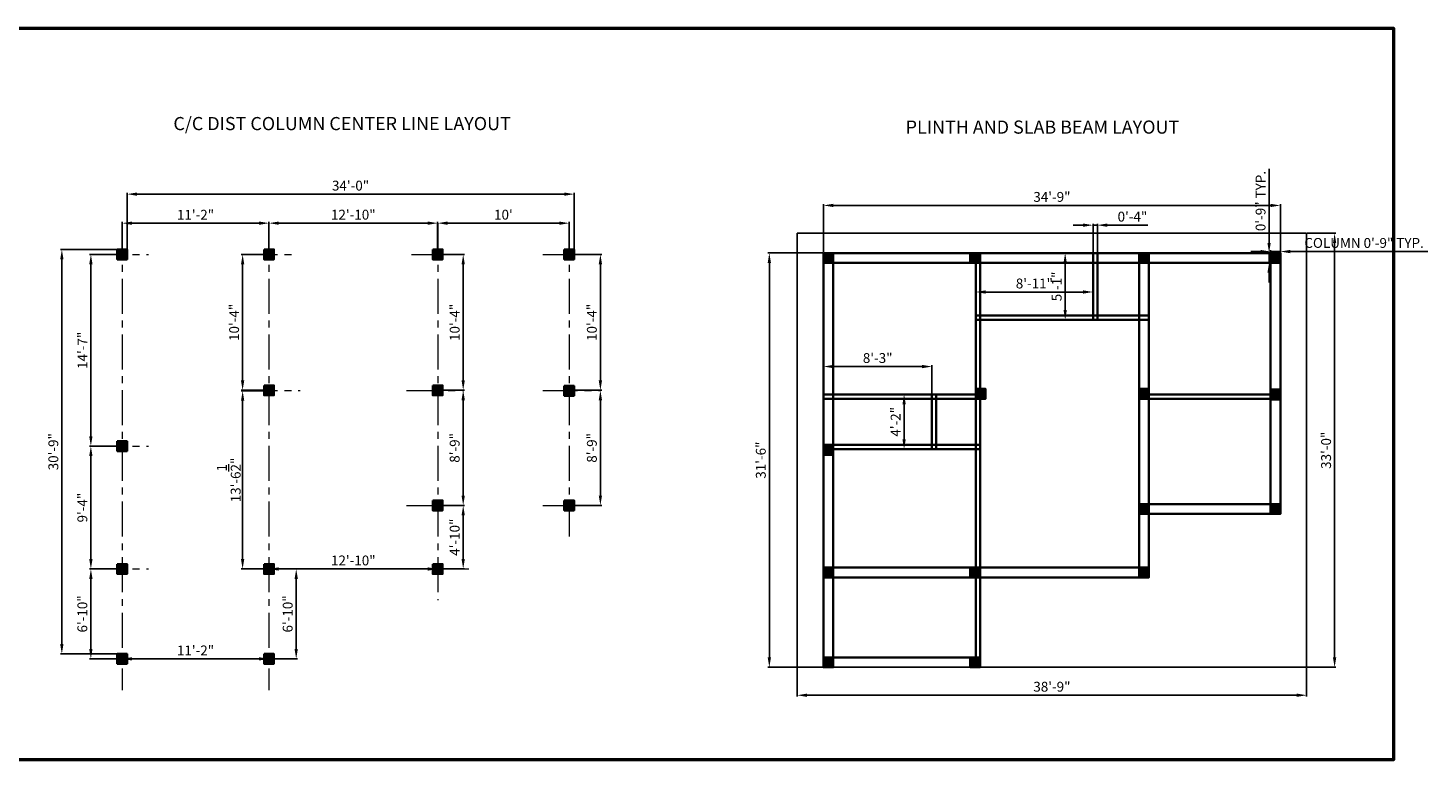
# Model space of a CAD drawing. Units: inches. Extents: x 2113 to 4530, y 1685 to 2353.
# Tile 6 of 6: x 3252 to 4530, y 1685 to 2353. Entities that reach past the tile are written whole.
import ezdxf

# ---------------------------------------------------------------- set-up
doc = ezdxf.new("R2010")
doc.units = ezdxf.units.IN
doc.linetypes.add('CENTER', pattern=[50.8, 31.75, -6.35, 6.35, -6.35])
for name, color, linetype, lineweight in [('A-ANNO-TITL', 7, 'Continuous', 35), ('A-ANNO-TTLB', 7, 'Continuous', 50), ('C-PROP', 7, 'Continuous', 25), ('S-ANNO-DIMS', 2, 'Continuous', 18), ('S-BEAM', 7, 'Continuous', 35), ('S-COLS', 1, 'Continuous', 35), ('S-COLS-PATT', 1, 'Continuous', 13), ('S-GRID', 8, 'CENTER', 18)]:
    doc.layers.add(name, color=color, linetype=linetype, lineweight=lineweight)
doc.styles.get("Standard").update_dxf_attribs({"font": 'arial.ttf'})
doc.dimstyles.new('ISO-25', dxfattribs={"dimtxt": 9, "dimasz": 9, "dimexe": 1.25, "dimexo": 0.625, "dimgap": 2, "dimtad": 1, "dimdec": 1, "dimlunit": 4, "dimtxsty": 'Standard', "dimcen": 2.5, "dimazin": 0, "dimtfac": 1, "dimtdec": 1, "dimtmove": 0, "dimatfit": 3, "dimfxl": 1, "dimarcsym": 0})

# ---------------------------------------------------------------- blocks, each defined once
blk = doc.blocks.new('*D9')
at = {"layer": 'Defpoints', "color": 0, "transparency": 16777216}
for p in [(3472, 2174.9), (3338, 2146.4), (3472, 2146.4)]:
    blk.add_point(p, dxfattribs=at)
at = {"layer": 'S-ANNO-DIMS', "color": 0, "lineweight": -2, "transparency": 16777216}
for p, q in [((3338, 2147), (3338, 2176.1)), ((3347, 2174.9), (3463, 2174.9)), ((3472, 2147), (3472, 2176.1))]:
    blk.add_line(p, q, dxfattribs=at)
at = {"layer": 'S-ANNO-DIMS', "color": 0, "transparency": 16777216}
for points in [[(3347, 2176.4), (3347, 2173.4), (3338, 2174.9)], [(3463, 2176.4), (3463, 2173.4), (3472, 2174.9)]]:
    blk.add_solid(points, dxfattribs=at)
at = {"layer": 'S-ANNO-DIMS', "color": 0, "transparency": 16777216, "insert": (3405, 2181.4), "char_height": 9, "attachment_point": 5}
blk.add_mtext('11\'-2"', dxfattribs=at)
blk = doc.blocks.new('*D10')
at = {"layer": 'Defpoints', "color": 0, "transparency": 16777216}
for p in [(3626, 2174.9), (3472, 2146.4), (3626, 2146.4)]:
    blk.add_point(p, dxfattribs=at)
at = {"layer": 'S-ANNO-DIMS', "color": 0, "lineweight": -2, "transparency": 16777216}
for p, q in [((3472, 2147), (3472, 2176.1)), ((3481, 2174.9), (3617, 2174.9)), ((3626, 2147), (3626, 2176.1))]:
    blk.add_line(p, q, dxfattribs=at)
at = {"layer": 'S-ANNO-DIMS', "color": 0, "transparency": 16777216}
for points in [[(3481, 2176.4), (3481, 2173.4), (3472, 2174.9)], [(3617, 2176.4), (3617, 2173.4), (3626, 2174.9)]]:
    blk.add_solid(points, dxfattribs=at)
at = {"layer": 'S-ANNO-DIMS', "color": 0, "transparency": 16777216, "insert": (3549, 2181.5), "char_height": 9, "attachment_point": 5}
blk.add_mtext('12\'-10"', dxfattribs=at)
blk = doc.blocks.new('*D11')
at = {"layer": 'Defpoints', "color": 0, "transparency": 16777216}
for p in [(3746, 2174.9), (3626, 2146.4), (3746, 2146.4)]:
    blk.add_point(p, dxfattribs=at)
at = {"layer": 'S-ANNO-DIMS', "color": 0, "lineweight": -2, "transparency": 16777216}
for p, q in [((3626, 2147), (3626, 2176.1)), ((3635, 2174.9), (3737, 2174.9)), ((3746, 2147), (3746, 2176.1))]:
    blk.add_line(p, q, dxfattribs=at)
at = {"layer": 'S-ANNO-DIMS', "color": 0, "transparency": 16777216}
for points in [[(3635, 2176.4), (3635, 2173.4), (3626, 2174.9)], [(3737, 2176.4), (3737, 2173.4), (3746, 2174.9)]]:
    blk.add_solid(points, dxfattribs=at)
at = {"layer": 'S-ANNO-DIMS', "color": 0, "transparency": 16777216, "insert": (3686, 2181.5), "char_height": 9, "attachment_point": 5}
blk.add_mtext("10'", dxfattribs=at)
blk = doc.blocks.new('*D12')
at = {"layer": 'Defpoints', "color": 0, "transparency": 16777216}
for p in [(3338, 2146.4), (3309.5, 1971.4), (3338, 1971.4)]:
    blk.add_point(p, dxfattribs=at)
at = {"layer": 'S-ANNO-DIMS', "color": 0, "lineweight": -2, "transparency": 16777216}
for p, q in [((3337.4, 2146.4), (3308.3, 2146.4)), ((3309.5, 2137.4), (3309.5, 1980.4)), ((3337.4, 1971.4), (3308.3, 1971.4))]:
    blk.add_line(p, q, dxfattribs=at)
at = {"layer": 'S-ANNO-DIMS', "color": 0, "transparency": 16777216}
for points in [[(3308, 2137.4), (3311, 2137.4), (3309.5, 2146.4)], [(3308, 1980.4), (3311, 1980.4), (3309.5, 1971.4)]]:
    blk.add_solid(points, dxfattribs=at)
at = {"layer": 'S-ANNO-DIMS', "color": 0, "transparency": 16777216, "insert": (3303, 2058.9), "char_height": 9, "attachment_point": 5, "rotation": 90}
blk.add_mtext('14\'-7"', dxfattribs=at)
blk = doc.blocks.new('*D13')
at = {"layer": 'Defpoints', "color": 0, "transparency": 16777216}
for p in [(3338, 1971.4), (3309.5, 1859.4), (3338, 1859.4)]:
    blk.add_point(p, dxfattribs=at)
at = {"layer": 'S-ANNO-DIMS', "color": 0, "lineweight": -2, "transparency": 16777216}
for p, q in [((3337.4, 1971.4), (3308.3, 1971.4)), ((3309.5, 1962.4), (3309.5, 1868.4)), ((3337.4, 1859.4), (3308.3, 1859.4))]:
    blk.add_line(p, q, dxfattribs=at)
at = {"layer": 'S-ANNO-DIMS', "color": 0, "transparency": 16777216}
for points in [[(3308, 1962.4), (3311, 1962.4), (3309.5, 1971.4)], [(3308, 1868.4), (3311, 1868.4), (3309.5, 1859.4)]]:
    blk.add_solid(points, dxfattribs=at)
at = {"layer": 'S-ANNO-DIMS', "color": 0, "transparency": 16777216, "insert": (3302.9, 1915.4), "char_height": 9, "attachment_point": 5, "rotation": 90}
blk.add_mtext('9\'-4"', dxfattribs=at)
blk = doc.blocks.new('*D14')
at = {"layer": 'Defpoints', "color": 0, "transparency": 16777216}
for p in [(3338, 1859.4), (3309.5, 1777.4), (3338, 1777.4)]:
    blk.add_point(p, dxfattribs=at)
at = {"layer": 'S-ANNO-DIMS', "color": 0, "lineweight": -2, "transparency": 16777216}
for p, q in [((3337.4, 1859.4), (3308.3, 1859.4)), ((3309.5, 1850.4), (3309.5, 1786.4)), ((3337.4, 1777.4), (3308.3, 1777.4))]:
    blk.add_line(p, q, dxfattribs=at)
at = {"layer": 'S-ANNO-DIMS', "color": 0, "transparency": 16777216}
for points in [[(3308, 1850.4), (3311, 1850.4), (3309.5, 1859.4)], [(3308, 1786.4), (3311, 1786.4), (3309.5, 1777.4)]]:
    blk.add_solid(points, dxfattribs=at)
at = {"layer": 'S-ANNO-DIMS', "color": 0, "transparency": 16777216, "insert": (3302.9, 1818.4), "char_height": 9, "attachment_point": 5, "rotation": 90}
blk.add_mtext('6\'-10"', dxfattribs=at)
blk = doc.blocks.new('*D15')
at = {"layer": 'Defpoints', "color": 0, "transparency": 16777216}
for p in [(3338, 1777.4), (3472, 1777.4), (3472, 1777.4)]:
    blk.add_point(p, dxfattribs=at)
at = {"layer": 'S-ANNO-DIMS', "color": 0, "lineweight": -2, "transparency": 16777216}
for p, q in [((3338, 1778), (3338, 1778.6)), ((3347, 1777.4), (3463, 1777.4)), ((3472, 1778), (3472, 1778.6))]:
    blk.add_line(p, q, dxfattribs=at)
at = {"layer": 'S-ANNO-DIMS', "color": 0, "transparency": 16777216}
for points in [[(3347, 1778.9), (3347, 1775.9), (3338, 1777.4)], [(3463, 1778.9), (3463, 1775.9), (3472, 1777.4)]]:
    blk.add_solid(points, dxfattribs=at)
at = {"layer": 'S-ANNO-DIMS', "color": 0, "transparency": 16777216, "insert": (3405, 1783.9), "char_height": 9, "attachment_point": 5}
blk.add_mtext('11\'-2"', dxfattribs=at)
blk = doc.blocks.new('*D16')
at = {"layer": 'Defpoints', "color": 0, "transparency": 16777216}
for p in [(3472, 1859.4), (3472, 1777.4), (3496.9, 1777.4)]:
    blk.add_point(p, dxfattribs=at)
at = {"layer": 'S-ANNO-DIMS', "color": 0, "lineweight": -2, "transparency": 16777216}
for p, q in [((3472.6, 1859.4), (3498.2, 1859.4)), ((3496.9, 1850.4), (3496.9, 1786.4)), ((3472.6, 1777.4), (3498.2, 1777.4))]:
    blk.add_line(p, q, dxfattribs=at)
at = {"layer": 'S-ANNO-DIMS', "color": 0, "transparency": 16777216}
for points in [[(3495.4, 1850.4), (3498.4, 1850.4), (3496.9, 1859.4)], [(3495.4, 1786.4), (3498.4, 1786.4), (3496.9, 1777.4)]]:
    blk.add_solid(points, dxfattribs=at)
at = {"layer": 'S-ANNO-DIMS', "color": 0, "transparency": 16777216, "insert": (3490.3, 1818.4), "char_height": 9, "attachment_point": 5, "rotation": 90}
blk.add_mtext('6\'-10"', dxfattribs=at)
blk = doc.blocks.new('*D17')
at = {"layer": 'Defpoints', "color": 0, "transparency": 16777216}
for p in [(3472, 1859.4), (3626, 1859.4), (3626, 1859.4)]:
    blk.add_point(p, dxfattribs=at)
at = {"layer": 'S-ANNO-DIMS', "color": 0, "lineweight": -2, "transparency": 16777216}
for p, q in [((3472, 1858.8), (3472, 1858.1)), ((3481, 1859.4), (3617, 1859.4)), ((3626, 1860), (3626, 1860.6))]:
    blk.add_line(p, q, dxfattribs=at)
at = {"layer": 'S-ANNO-DIMS', "color": 0, "transparency": 16777216}
for points in [[(3481, 1860.9), (3481, 1857.9), (3472, 1859.4)], [(3617, 1860.9), (3617, 1857.9), (3626, 1859.4)]]:
    blk.add_solid(points, dxfattribs=at)
at = {"layer": 'S-ANNO-DIMS', "color": 0, "transparency": 16777216, "insert": (3549, 1866), "char_height": 9, "attachment_point": 5}
blk.add_mtext('12\'-10"', dxfattribs=at)
blk = doc.blocks.new('*D18')
at = {"layer": 'Defpoints', "color": 0, "transparency": 16777216}
for p in [(3626, 1917.4), (3626, 1859.4), (3649.3, 1859.4)]:
    blk.add_point(p, dxfattribs=at)
at = {"layer": 'S-ANNO-DIMS', "color": 0, "lineweight": -2, "transparency": 16777216}
for p, q in [((3626.6, 1917.4), (3650.5, 1917.4)), ((3649.3, 1908.4), (3649.3, 1868.4)), ((3626.6, 1859.4), (3650.5, 1859.4))]:
    blk.add_line(p, q, dxfattribs=at)
at = {"layer": 'S-ANNO-DIMS', "color": 0, "transparency": 16777216}
for points in [[(3647.8, 1908.4), (3650.8, 1908.4), (3649.3, 1917.4)], [(3647.8, 1868.4), (3650.8, 1868.4), (3649.3, 1859.4)]]:
    blk.add_solid(points, dxfattribs=at)
at = {"layer": 'S-ANNO-DIMS', "color": 0, "transparency": 16777216, "insert": (3642.7, 1888.4), "char_height": 9, "attachment_point": 5, "rotation": 90}
blk.add_mtext('4\'-10"', dxfattribs=at)
blk = doc.blocks.new('*D19')
at = {"layer": 'Defpoints', "color": 0, "transparency": 16777216}
for p in [(3626, 2022.4), (3626, 1917.4), (3649.3, 1917.4)]:
    blk.add_point(p, dxfattribs=at)
at = {"layer": 'S-ANNO-DIMS', "color": 0, "lineweight": -2, "transparency": 16777216}
for p, q in [((3626.6, 2022.4), (3650.5, 2022.4)), ((3649.3, 2013.4), (3649.3, 1926.4)), ((3626.6, 1917.4), (3650.5, 1917.4))]:
    blk.add_line(p, q, dxfattribs=at)
at = {"layer": 'S-ANNO-DIMS', "color": 0, "transparency": 16777216}
for points in [[(3647.8, 2013.4), (3650.8, 2013.4), (3649.3, 2022.4)], [(3647.8, 1926.4), (3650.8, 1926.4), (3649.3, 1917.4)]]:
    blk.add_solid(points, dxfattribs=at)
at = {"layer": 'S-ANNO-DIMS', "color": 0, "transparency": 16777216, "insert": (3642.7, 1969.9), "char_height": 9, "attachment_point": 5, "rotation": 90}
blk.add_mtext('8\'-9"', dxfattribs=at)
blk = doc.blocks.new('*D20')
at = {"layer": 'Defpoints', "color": 0, "transparency": 16777216}
for p in [(3626, 2146.4), (3626, 2022.4), (3649.3, 2022.4)]:
    blk.add_point(p, dxfattribs=at)
at = {"layer": 'S-ANNO-DIMS', "color": 0, "lineweight": -2, "transparency": 16777216}
for p, q in [((3626.6, 2146.4), (3650.5, 2146.4)), ((3649.3, 2137.4), (3649.3, 2031.4)), ((3626.6, 2022.4), (3650.5, 2022.4))]:
    blk.add_line(p, q, dxfattribs=at)
at = {"layer": 'S-ANNO-DIMS', "color": 0, "transparency": 16777216}
for points in [[(3647.8, 2137.4), (3650.8, 2137.4), (3649.3, 2146.4)], [(3647.8, 2031.4), (3650.8, 2031.4), (3649.3, 2022.4)]]:
    blk.add_solid(points, dxfattribs=at)
at = {"layer": 'S-ANNO-DIMS', "color": 0, "transparency": 16777216, "insert": (3642.7, 2084.4), "char_height": 9, "attachment_point": 5, "rotation": 90}
blk.add_mtext('10\'-4"', dxfattribs=at)
blk = doc.blocks.new('*D21')
at = {"layer": 'Defpoints', "color": 0, "transparency": 16777216}
for p in [(3472, 2146.4), (3448, 2022.4), (3472, 2022.4)]:
    blk.add_point(p, dxfattribs=at)
at = {"layer": 'S-ANNO-DIMS', "color": 0, "lineweight": -2, "transparency": 16777216}
for p, q in [((3471.4, 2146.4), (3446.8, 2146.4)), ((3448, 2137.4), (3448, 2031.4)), ((3471.4, 2022.4), (3446.8, 2022.4))]:
    blk.add_line(p, q, dxfattribs=at)
at = {"layer": 'S-ANNO-DIMS', "color": 0, "transparency": 16777216}
for points in [[(3446.5, 2137.4), (3449.5, 2137.4), (3448, 2146.4)], [(3446.5, 2031.4), (3449.5, 2031.4), (3448, 2022.4)]]:
    blk.add_solid(points, dxfattribs=at)
at = {"layer": 'S-ANNO-DIMS', "color": 0, "transparency": 16777216, "insert": (3441.4, 2084.4), "char_height": 9, "attachment_point": 5, "rotation": 90}
blk.add_mtext('10\'-4"', dxfattribs=at)
blk = doc.blocks.new('*D22')
at = {"layer": 'Defpoints', "color": 0, "transparency": 16777216}
for p in [(3471.5, 2021.9), (3448, 1859.4), (3472, 1859.4)]:
    blk.add_point(p, dxfattribs=at)
at = {"layer": 'S-ANNO-DIMS', "color": 0, "lineweight": -2, "transparency": 16777216}
for p, q in [((3470.9, 2021.9), (3446.8, 2021.9)), ((3448, 2012.9), (3448, 1868.4)), ((3471.4, 1859.4), (3446.8, 1859.4))]:
    blk.add_line(p, q, dxfattribs=at)
at = {"layer": 'S-ANNO-DIMS', "color": 0, "transparency": 16777216}
for points in [[(3446.5, 2012.9), (3449.5, 2012.9), (3448, 2021.9)], [(3446.5, 1868.4), (3449.5, 1868.4), (3448, 1859.4)]]:
    blk.add_solid(points, dxfattribs=at)
at = {"layer": 'S-ANNO-DIMS', "color": 0, "transparency": 16777216, "insert": (3435.4, 1940.6), "char_height": 9, "attachment_point": 5, "rotation": 90}
blk.add_mtext('13\'-6{\\H1x;\\S1/2;}"', dxfattribs=at)
blk = doc.blocks.new('*D23')
at = {"layer": 'Defpoints', "color": 0, "transparency": 16777216}
for p in [(3746, 2146.4), (3746, 2022.4), (3774.5, 2022.4)]:
    blk.add_point(p, dxfattribs=at)
at = {"layer": 'S-ANNO-DIMS', "color": 0, "lineweight": -2, "transparency": 16777216}
for p, q in [((3746.6, 2146.4), (3775.8, 2146.4)), ((3774.5, 2137.4), (3774.5, 2031.4)), ((3746.6, 2022.4), (3775.8, 2022.4))]:
    blk.add_line(p, q, dxfattribs=at)
at = {"layer": 'S-ANNO-DIMS', "color": 0, "transparency": 16777216}
for points in [[(3773, 2137.4), (3776, 2137.4), (3774.5, 2146.4)], [(3773, 2031.4), (3776, 2031.4), (3774.5, 2022.4)]]:
    blk.add_solid(points, dxfattribs=at)
at = {"layer": 'S-ANNO-DIMS', "color": 0, "transparency": 16777216, "insert": (3767.9, 2084.4), "char_height": 9, "attachment_point": 5, "rotation": 90}
blk.add_mtext('10\'-4"', dxfattribs=at)
blk = doc.blocks.new('*D24')
at = {"layer": 'Defpoints', "color": 0, "transparency": 16777216}
for p in [(3746, 2022.4), (3746, 1917.4), (3774.5, 1917.4)]:
    blk.add_point(p, dxfattribs=at)
at = {"layer": 'S-ANNO-DIMS', "color": 0, "lineweight": -2, "transparency": 16777216}
for p, q in [((3746.6, 2022.4), (3775.8, 2022.4)), ((3774.5, 2013.4), (3774.5, 1926.4)), ((3746.6, 1917.4), (3775.8, 1917.4))]:
    blk.add_line(p, q, dxfattribs=at)
at = {"layer": 'S-ANNO-DIMS', "color": 0, "transparency": 16777216}
for points in [[(3773, 2013.4), (3776, 2013.4), (3774.5, 2022.4)], [(3773, 1926.4), (3776, 1926.4), (3774.5, 1917.4)]]:
    blk.add_solid(points, dxfattribs=at)
at = {"layer": 'S-ANNO-DIMS', "color": 0, "transparency": 16777216, "insert": (3767.9, 1969.9), "char_height": 9, "attachment_point": 5, "rotation": 90}
blk.add_mtext('8\'-9"', dxfattribs=at)
blk = doc.blocks.new('COL-9X9')
h = blk.add_hatch(color=256)
h.dxf.hatch_style = 1
h.paths.add_polyline_path([(9, 0), (9, 9), (0, 9), (0, 0)])
blk.add_lwpolyline([(0, 9), (9, 9), (9, 0), (0, 0)], close=True)
blk = doc.blocks.new('LOT-465X396')
for p, q in [((0, 396), (465, 396)), ((0, 396), (0, 0)), ((465, 396), (465, 0)), ((0, 0), (465, 0))]:
    blk.add_line(p, q)
blk = doc.blocks.new('*D38')
at = {"layer": 'Defpoints', "color": 0, "transparency": 16777216}
for p in [(4386.1, 2147.7), (4395.1, 2149), (4395.1, 2147.7)]:
    blk.add_point(p, dxfattribs=at)
at = {"layer": 'S-ANNO-DIMS', "color": 0, "lineweight": -2, "transparency": 16777216}
for p, q in [((4377.1, 2149), (4368.1, 2149)), ((4386.1, 2148.3), (4386.1, 2150.3)), ((4386.1, 2149), (4395.1, 2149)), ((4395.1, 2148.3), (4395.1, 2150.3)), ((4404.1, 2149), (4529.8, 2149))]:
    blk.add_line(p, q, dxfattribs=at)
at = {"layer": 'S-ANNO-DIMS', "color": 0, "transparency": 16777216}
for points in [[(4377.1, 2150.5), (4377.1, 2147.5), (4386.1, 2149)], [(4404.1, 2150.5), (4404.1, 2147.5), (4395.1, 2149)]]:
    blk.add_solid(points, dxfattribs=at)
at = {"layer": 'S-ANNO-DIMS', "color": 0, "transparency": 16777216, "insert": (4471.5, 2155.7), "char_height": 9, "attachment_point": 5}
blk.add_mtext('COLUMN 0\'-9" TYP.', dxfattribs=at)
blk = doc.blocks.new('*D39')
at = {"layer": 'Defpoints', "color": 0, "transparency": 16777216}
for p in [(4384.8, 2147.7), (4386.1, 2147.7), (4386.1, 2138.7)]:
    blk.add_point(p, dxfattribs=at)
at = {"layer": 'S-ANNO-DIMS', "color": 0, "lineweight": -2, "transparency": 16777216}
for p, q in [((4384.8, 2156.7), (4384.8, 2224.5)), ((4385.5, 2147.7), (4383.5, 2147.7)), ((4384.8, 2138.7), (4384.8, 2147.7)), ((4385.5, 2138.7), (4383.5, 2138.7)), ((4384.8, 2129.7), (4384.8, 2120.7))]:
    blk.add_line(p, q, dxfattribs=at)
at = {"layer": 'S-ANNO-DIMS', "color": 0, "transparency": 16777216}
for points in [[(4383.3, 2156.7), (4386.3, 2156.7), (4384.8, 2147.7)], [(4383.3, 2129.7), (4386.3, 2129.7), (4384.8, 2138.7)]]:
    blk.add_solid(points, dxfattribs=at)
at = {"layer": 'S-ANNO-DIMS', "color": 0, "transparency": 16777216, "insert": (4378.2, 2195.1), "char_height": 9, "attachment_point": 5, "rotation": 90}
blk.add_mtext('0\'-9" TYP.', dxfattribs=at)
blk = doc.blocks.new('*D79')
at = {"layer": 'Defpoints', "color": 0, "transparency": 16777216}
for p in [(3283, 2150.9), (3342.5, 2150.9), (3342.5, 1781.9)]:
    blk.add_point(p, dxfattribs=at)
at = {"layer": 'S-ANNO-DIMS', "color": 0, "lineweight": -2, "transparency": 16777216}
for p, q in [((3341.9, 2150.9), (3281.7, 2150.9)), ((3283, 1790.9), (3283, 2141.9)), ((3341.9, 1781.9), (3281.7, 1781.9))]:
    blk.add_line(p, q, dxfattribs=at)
at = {"layer": 'S-ANNO-DIMS', "color": 0, "transparency": 16777216}
for points in [[(3281.5, 2141.9), (3284.5, 2141.9), (3283, 2150.9)], [(3281.5, 1790.9), (3284.5, 1790.9), (3283, 1781.9)]]:
    blk.add_solid(points, dxfattribs=at)
at = {"layer": 'S-ANNO-DIMS', "color": 0, "transparency": 16777216, "insert": (3276.4, 1966.4), "char_height": 9, "attachment_point": 5, "rotation": 90}
blk.add_mtext('30\'-9"', dxfattribs=at)
blk = doc.blocks.new('*D80')
at = {"layer": 'Defpoints', "color": 0, "transparency": 16777216}
for p in [(3750.5, 2201.4), (3342.5, 2150.9), (3750.5, 2146.4)]:
    blk.add_point(p, dxfattribs=at)
at = {"layer": 'S-ANNO-DIMS', "color": 0, "lineweight": -2, "transparency": 16777216}
for p, q in [((3342.5, 2151.5), (3342.5, 2202.7)), ((3351.5, 2201.4), (3741.5, 2201.4)), ((3750.5, 2147), (3750.5, 2202.7))]:
    blk.add_line(p, q, dxfattribs=at)
at = {"layer": 'S-ANNO-DIMS', "color": 0, "transparency": 16777216}
for points in [[(3351.5, 2202.9), (3351.5, 2199.9), (3342.5, 2201.4)], [(3741.5, 2202.9), (3741.5, 2199.9), (3750.5, 2201.4)]]:
    blk.add_solid(points, dxfattribs=at)
at = {"layer": 'S-ANNO-DIMS', "color": 0, "transparency": 16777216, "insert": (3546.5, 2208), "char_height": 9, "attachment_point": 5}
blk.add_mtext('34\'-0"', dxfattribs=at)
blk = doc.blocks.new('*D81')
at = {"layer": 'Defpoints', "color": 0, "transparency": 16777216}
for p in [(4224.1, 2112.1), (4117.1, 2086.7), (4224.1, 2086.7)]:
    blk.add_point(p, dxfattribs=at)
at = {"layer": 'S-ANNO-DIMS', "color": 0, "lineweight": -2, "transparency": 16777216}
for p, q in [((4117.1, 2087.3), (4117.1, 2113.4)), ((4126.1, 2112.1), (4215.1, 2112.1)), ((4224.1, 2087.3), (4224.1, 2113.4))]:
    blk.add_line(p, q, dxfattribs=at)
at = {"layer": 'S-ANNO-DIMS', "color": 0, "transparency": 16777216}
for points in [[(4126.1, 2113.6), (4126.1, 2110.6), (4117.1, 2112.1)], [(4215.1, 2113.6), (4215.1, 2110.6), (4224.1, 2112.1)]]:
    blk.add_solid(points, dxfattribs=at)
at = {"layer": 'S-ANNO-DIMS', "color": 0, "transparency": 16777216, "insert": (4170.6, 2118.7), "char_height": 9, "attachment_point": 5}
blk.add_mtext('8\'-11"', dxfattribs=at)
blk = doc.blocks.new('*D82')
at = {"layer": 'Defpoints', "color": 0, "transparency": 16777216}
for p in [(4198.7, 2147.7), (4224.1, 2147.7), (4224.1, 2086.7)]:
    blk.add_point(p, dxfattribs=at)
at = {"layer": 'S-ANNO-DIMS', "color": 0, "lineweight": -2, "transparency": 16777216}
for p, q in [((4223.5, 2147.7), (4197.4, 2147.7)), ((4198.7, 2095.7), (4198.7, 2138.7)), ((4223.5, 2086.7), (4197.4, 2086.7))]:
    blk.add_line(p, q, dxfattribs=at)
at = {"layer": 'S-ANNO-DIMS', "color": 0, "transparency": 16777216}
for points in [[(4197.2, 2138.7), (4200.2, 2138.7), (4198.7, 2147.7)], [(4197.2, 2095.7), (4200.2, 2095.7), (4198.7, 2086.7)]]:
    blk.add_solid(points, dxfattribs=at)
at = {"layer": 'S-ANNO-DIMS', "color": 0, "transparency": 16777216, "insert": (4192.1, 2117.2), "char_height": 9, "attachment_point": 5, "rotation": 90}
blk.add_mtext('5\'-1"', dxfattribs=at)
blk = doc.blocks.new('*D83')
at = {"layer": 'Defpoints', "color": 0, "transparency": 16777216}
for p in [(4077.1, 2044.1), (3978.1, 2018.7), (4077.1, 2018.7)]:
    blk.add_point(p, dxfattribs=at)
at = {"layer": 'S-ANNO-DIMS', "color": 0, "lineweight": -2, "transparency": 16777216}
for p, q in [((3978.1, 2019.3), (3978.1, 2045.4)), ((4077.1, 2019.3), (4077.1, 2045.4)), ((3987.1, 2044.1), (4068.1, 2044.1))]:
    blk.add_line(p, q, dxfattribs=at)
at = {"layer": 'S-ANNO-DIMS', "color": 0, "transparency": 16777216}
for points in [[(3987.1, 2045.6), (3987.1, 2042.6), (3978.1, 2044.1)], [(4068.1, 2045.6), (4068.1, 2042.6), (4077.1, 2044.1)]]:
    blk.add_solid(points, dxfattribs=at)
at = {"layer": 'S-ANNO-DIMS', "color": 0, "transparency": 16777216, "insert": (4027.6, 2050.7), "char_height": 9, "attachment_point": 5}
blk.add_mtext('8\'-3"', dxfattribs=at)
blk = doc.blocks.new('*D84')
at = {"layer": 'Defpoints', "color": 0, "transparency": 16777216}
for p in [(4051.7, 2018.7), (4077.1, 2018.7), (4077.1, 1968.7)]:
    blk.add_point(p, dxfattribs=at)
at = {"layer": 'S-ANNO-DIMS', "color": 0, "lineweight": -2, "transparency": 16777216}
for p, q in [((4076.5, 2018.7), (4050.4, 2018.7)), ((4051.7, 1977.7), (4051.7, 2009.7)), ((4076.5, 1968.7), (4050.4, 1968.7))]:
    blk.add_line(p, q, dxfattribs=at)
at = {"layer": 'S-ANNO-DIMS', "color": 0, "transparency": 16777216}
for points in [[(4050.2, 2009.7), (4053.2, 2009.7), (4051.7, 2018.7)], [(4050.2, 1977.7), (4053.2, 1977.7), (4051.7, 1968.7)]]:
    blk.add_solid(points, dxfattribs=at)
at = {"layer": 'S-ANNO-DIMS', "color": 0, "transparency": 16777216, "insert": (4045.1, 1993.7), "char_height": 9, "attachment_point": 5, "rotation": 90}
blk.add_mtext('4\'-2"', dxfattribs=at)
blk = doc.blocks.new('*D85')
at = {"layer": 'Defpoints', "color": 0, "transparency": 16777216}
for p in [(4228.1, 2173.1), (4224.1, 2147.7), (4228.1, 2147.7)]:
    blk.add_point(p, dxfattribs=at)
at = {"layer": 'S-ANNO-DIMS', "color": 0, "lineweight": -2, "transparency": 16777216}
for p, q in [((4215.1, 2173.1), (4206.1, 2173.1)), ((4224.1, 2148.3), (4224.1, 2174.4)), ((4224.1, 2173.1), (4228.1, 2173.1)), ((4228.1, 2148.3), (4228.1, 2174.4)), ((4237.1, 2173.1), (4274, 2173.1))]:
    blk.add_line(p, q, dxfattribs=at)
at = {"layer": 'S-ANNO-DIMS', "color": 0, "transparency": 16777216}
for points in [[(4215.1, 2174.6), (4215.1, 2171.6), (4224.1, 2173.1)], [(4237.1, 2174.6), (4237.1, 2171.6), (4228.1, 2173.1)]]:
    blk.add_solid(points, dxfattribs=at)
at = {"layer": 'S-ANNO-DIMS', "color": 0, "transparency": 16777216, "insert": (4260.1, 2179.7), "char_height": 9, "attachment_point": 5}
blk.add_mtext('0\'-4"', dxfattribs=at)
blk = doc.blocks.new('*D86')
at = {"layer": 'Defpoints', "color": 0, "transparency": 16777216}
for p in [(4395.1, 2191.1), (3978.1, 2147.7), (4395.1, 2147.7)]:
    blk.add_point(p, dxfattribs=at)
at = {"layer": 'S-ANNO-DIMS', "color": 0, "lineweight": -2, "transparency": 16777216}
for p, q in [((3978.1, 2148.3), (3978.1, 2192.4)), ((3987.1, 2191.1), (4386.1, 2191.1)), ((4395.1, 2148.3), (4395.1, 2192.4))]:
    blk.add_line(p, q, dxfattribs=at)
at = {"layer": 'S-ANNO-DIMS', "color": 0, "transparency": 16777216}
for points in [[(3987.1, 2192.6), (3987.1, 2189.6), (3978.1, 2191.1)], [(4386.1, 2192.6), (4386.1, 2189.6), (4395.1, 2191.1)]]:
    blk.add_solid(points, dxfattribs=at)
at = {"layer": 'S-ANNO-DIMS', "color": 0, "transparency": 16777216, "insert": (4186.6, 2197.7), "char_height": 9, "attachment_point": 5}
blk.add_mtext('34\'-9"', dxfattribs=at)
blk = doc.blocks.new('*D87')
at = {"layer": 'Defpoints', "color": 0, "transparency": 16777216}
for p in [(3928.7, 2147.7), (3978.1, 2147.7), (3978.1, 1769.7)]:
    blk.add_point(p, dxfattribs=at)
at = {"layer": 'S-ANNO-DIMS', "color": 0, "lineweight": -2, "transparency": 16777216}
for p, q in [((3977.5, 2147.7), (3927.4, 2147.7)), ((3928.7, 1778.7), (3928.7, 2138.7)), ((3977.5, 1769.7), (3927.4, 1769.7))]:
    blk.add_line(p, q, dxfattribs=at)
at = {"layer": 'S-ANNO-DIMS', "color": 0, "transparency": 16777216}
for points in [[(3927.2, 2138.7), (3930.2, 2138.7), (3928.7, 2147.7)], [(3927.2, 1778.7), (3930.2, 1778.7), (3928.7, 1769.7)]]:
    blk.add_solid(points, dxfattribs=at)
at = {"layer": 'S-ANNO-DIMS', "color": 0, "transparency": 16777216, "insert": (3922.1, 1958.7), "char_height": 9, "attachment_point": 5, "rotation": 90}
blk.add_mtext('31\'-6"', dxfattribs=at)
blk = doc.blocks.new('*D88')
at = {"layer": 'Defpoints', "color": 0, "transparency": 16777216}
for p in [(3954.1, 1769.7), (4419.1, 1769.7), (4419.1, 1744.2)]:
    blk.add_point(p, dxfattribs=at)
at = {"layer": 'S-ANNO-DIMS', "color": 0, "lineweight": -2, "transparency": 16777216}
for p, q in [((3954.1, 1769.1), (3954.1, 1743)), ((4419.1, 1769.1), (4419.1, 1743)), ((3963.1, 1744.2), (4410.1, 1744.2))]:
    blk.add_line(p, q, dxfattribs=at)
at = {"layer": 'S-ANNO-DIMS', "color": 0, "transparency": 16777216}
for points in [[(3963.1, 1745.7), (3963.1, 1742.7), (3954.1, 1744.2)], [(4410.1, 1745.7), (4410.1, 1742.7), (4419.1, 1744.2)]]:
    blk.add_solid(points, dxfattribs=at)
at = {"layer": 'S-ANNO-DIMS', "color": 0, "transparency": 16777216, "insert": (4186.6, 1750.8), "char_height": 9, "attachment_point": 5}
blk.add_mtext('38\'-9"', dxfattribs=at)
blk = doc.blocks.new('*D89')
at = {"layer": 'Defpoints', "color": 0, "transparency": 16777216}
for p in [(4419.1, 2165.7), (4419.1, 1769.7), (4444.6, 1769.7)]:
    blk.add_point(p, dxfattribs=at)
at = {"layer": 'S-ANNO-DIMS', "color": 0, "lineweight": -2, "transparency": 16777216}
for p, q in [((4419.7, 2165.7), (4445.8, 2165.7)), ((4444.6, 2156.7), (4444.6, 1778.7)), ((4419.7, 1769.7), (4445.8, 1769.7))]:
    blk.add_line(p, q, dxfattribs=at)
at = {"layer": 'S-ANNO-DIMS', "color": 0, "transparency": 16777216}
for points in [[(4443.1, 2156.7), (4446.1, 2156.7), (4444.6, 2165.7)], [(4443.1, 1778.7), (4446.1, 1778.7), (4444.6, 1769.7)]]:
    blk.add_solid(points, dxfattribs=at)
at = {"layer": 'S-ANNO-DIMS', "color": 0, "transparency": 16777216, "insert": (4438, 1967.7), "char_height": 9, "attachment_point": 5, "rotation": 90}
blk.add_mtext('33\'-0"', dxfattribs=at)

msp = doc.modelspace()

# ---------------------------------------------------------------- hatches: boundary and pattern name
at = {"layer": 'S-COLS-PATT'}
h = msp.add_hatch(color=256, dxfattribs=at)
h.dxf.hatch_style = 1
h.paths.add_polyline_path([(3476.51, 2026.89), (3467.51, 2026.89), (3467.51, 2017.89), (3476.51, 2017.89)])

# ---------------------------------------------------------------- linework, layer by layer
at = {"layer": 'A-ANNO-TTLB'}
msp.add_lwpolyline([(2112.77, 2352.97), (4498.42, 2352.97), (4498.42, 1685.12), (2112.77, 1685.12)], close=True, dxfattribs=at)
at = {"layer": 'S-BEAM'}
for p, q in [((3978.1, 2147.68), (4395.1, 2147.68)), ((3978.1, 2147.68), (3978.1, 1769.68)), ((3987.1, 2147.68), (3987.1, 1769.68)), ((4117.1, 2147.68), (4117.1, 1968.68)), ((4121.1, 2147.68), (4121.1, 2018.68)), ((4224.1, 2147.68), (4224.1, 2086.68)), ((4228.1, 2147.68), (4228.1, 2090.68)), ((4266.1, 2147.68), (4266.1, 1976.68)), ((4275.1, 2147.68), (4275.1, 1976.68)), ((4386.1, 2147.68), (4386.1, 1909.68)), ((4395.1, 2147.68), (4395.1, 1909.68)), ((3978.1, 2138.68), (4395.1, 2138.68)), ((4117.1, 2090.68), (4275.1, 2090.68)), ((4117.1, 2086.68), (4275.1, 2086.68)), ((4121.1, 2086.68), (4121.1, 2014.68)), ((4224.1, 2092.68), (4224.1, 2090.68)), ((4228.1, 2092.68), (4228.1, 2086.68)), ((3978.1, 2018.68), (4121.1, 2018.68)), ((3978.1, 2014.68), (4121.1, 2014.68)), ((3987.1, 2018.68), (4039.1, 2018.68)), ((3987.1, 2014.68), (4039.1, 2014.68)), ((4075.1, 2018.68), (4081.1, 2018.68)), ((4075.1, 2018.68), (4081.1, 2018.68)), ((4077.1, 2018.68), (4077.1, 1968.68)), ((4077.1, 2014.68), (4081.1, 2014.68)), ((4081.1, 2018.68), (4081.1, 1968.68)), ((4115.1, 2018.68), (4117.1, 2018.68)), ((4115.1, 2014.68), (4121.1, 2014.68)), ((4117.1, 2018.68), (4117.1, 2014.68)), ((4117.1, 2014.68), (4121.1, 2014.68)), ((4117.1, 2014.68), (4117.1, 1769.68)), ((4121.1, 2018.68), (4121.1, 1860.68)), ((4266.1, 2018.68), (4395.1, 2018.68)), ((4266.1, 2018.68), (4266.1, 2014.68)), ((4266.1, 2014.68), (4395.1, 2014.68)), ((3978.1, 1972.68), (4117.1, 1972.68)), ((3978.1, 1968.68), (4117.1, 1968.68)), ((4115.1, 1972.68), (4121.1, 1972.68)), ((4117.1, 1968.68), (4121.1, 1968.68)), ((4266.1, 1976.68), (4266.1, 1851.68)), ((4275.1, 1976.68), (4275.1, 1860.68)), ((4266.1, 1918.68), (4395.1, 1918.68)), ((4276.1, 1918.68), (4300.1, 1918.68)), ((4266.1, 1909.68), (4395.1, 1909.68)), ((3978.1, 1860.68), (4117.1, 1860.68)), ((3987.1, 1860.68), (4275.1, 1860.68)), ((4121.1, 1860.68), (4121.1, 1769.68)), ((4275.1, 1862.68), (4275.1, 1851.68)), ((3978.1, 1851.68), (4275.1, 1851.68)), ((3978.1, 1778.68), (4121.1, 1778.68))]:
    msp.add_line(p, q, dxfattribs=at)
at = {"layer": 'S-COLS'}
for p, q in [((3470.51, 2026.89), (3476.51, 2026.89)), ((3470.51, 2021.89), (3472.51, 2021.89)), ((3621.51, 2021.89), (3621.51, 2017.89)), ((3630.51, 1863.89), (3630.51, 1854.89))]:
    msp.add_line(p, q, dxfattribs=at)
msp.add_lwpolyline([(3467.51, 2026.89), (3476.51, 2026.89), (3476.51, 2017.89), (3467.51, 2017.89)], close=True, dxfattribs=at)
at = {"layer": 'S-GRID'}
for p, q in [((3338.01, 2174.89), (3338.01, 1748.89)), ((3472.01, 2174.89), (3472.01, 1748.89)), ((3626.01, 2174.89), (3626.01, 1830.89)), ((3746.01, 2174.89), (3746.01, 1888.89)), ((3309.51, 2146.39), (3362.01, 2146.39)), ((3448.01, 2146.39), (3496.01, 2146.39)), ((3602.01, 2146.39), (3650.01, 2146.39)), ((3722.01, 2146.39), (3750.51, 2146.39)), ((3448.01, 2022.39), (3500.51, 2022.39)), ((3597.51, 2022.39), (3650.01, 2022.39)), ((3722.01, 2022.39), (3774.51, 2022.39)), ((3309.51, 1971.39), (3362.01, 1971.39)), ((3597.51, 1917.39), (3650.01, 1917.39)), ((3722.01, 1917.39), (3774.51, 1917.39)), ((3309.51, 1859.39), (3362.01, 1859.39)), ((3448.01, 1859.39), (3496.01, 1859.39)), ((3597.51, 1859.39), (3654.51, 1859.39)), ((3309.51, 1777.39), (3362.01, 1777.39)), ((3448.01, 1777.39), (3496.01, 1777.39))]:
    msp.add_line(p, q, dxfattribs=at)

# ---------------------------------------------------------------- block references
at = {"layer": 'C-PROP', "rotation": 180}
msp.add_blockref('LOT-465X396', (4419.1, 2165.68), dxfattribs=at)
at = {"layer": 'S-COLS'}
for p in [(3333.51, 2141.89), (3467.51, 2141.89), (3621.51, 2141.89), (3741.51, 2141.89), (3978.1, 2138.68), (4112.1, 2138.68), (4266.1, 2138.68), (4386.1, 2138.68), (3621.51, 2017.89), (3741.51, 2017.39), (4117.1, 2014.68), (4266.1, 2014.68), (4386.1, 2014.18), (3333.51, 1966.89), (3978.1, 1963.68), (3621.51, 1912.89), (3741.51, 1912.89), (4266.1, 1909.68), (4386.1, 1909.68), (3333.51, 1854.89), (3467.51, 1854.89), (3621.51, 1854.89), (3978.1, 1851.68), (4112.1, 1851.68), (4266.1, 1851.68), (3333.51, 1772.89), (3467.51, 1772.89), (3978.1, 1769.68), (4112.1, 1769.68)]:
    msp.add_blockref('COL-9X9', p, dxfattribs=at)

# ---------------------------------------------------------------- texts
at = {"layer": 'A-ANNO-TITL'}
for s, p in [('C/C DIST COLUMN CENTER LINE LAYOUT', (3384.81, 2259.78)), ('PLINTH AND SLAB BEAM LAYOUT', (4053.14, 2256.57))]:
    msp.add_text(s, height=12, dxfattribs=at).set_placement(p)

# ---------------------------------------------------------------- dimensions: what is measured, and where the dimension line sits
at = {"layer": 'S-ANNO-DIMS'}
dim = msp.add_linear_dim(base=(4384.75, 2147.68), p1=(4386.1, 2138.68), p2=(4386.1, 2147.68), angle=90, text='<> TYP.', dimstyle='ISO-25', override={"dimdec": 1, "dimlfac": 1, "dimrnd": 0, "dimzin": 1, "dimdsep": 46, "dimlunit": 4, "dimfrac": 2}, dxfattribs=at)
dim.commit()
dim.dimension.update_dxf_attribs({"geometry": '*D39', "text_midpoint": (4378.16, 2195.11)})
for base, p1, p2, override, picture, middle in [((3750.51, 2201.44), (3342.51, 2150.89), (3750.51, 2146.39), {"dimdec": 1, "dimlfac": 1, "dimrnd": 0, "dimzin": 1, "dimdsep": 46, "dimlunit": 4, "dimfrac": 2}, '*D80', (3546.51, 2208.03)), ((4395.1, 2191.13), (3978.1, 2147.68), (4395.1, 2147.68), {"dimdec": 1, "dimlfac": 1, "dimrnd": 0, "dimzin": 1, "dimdsep": 46, "dimlunit": 4, "dimfrac": 2}, '*D86', (4186.6, 2197.73)), ((3472.01, 2174.89), (3338.01, 2146.39), (3472.01, 2146.39), {"dimclrd": 0, "dimclre": 0, "dimclrt": 0}, '*D9', (3405.01, 2181.4)), ((3626.01, 2174.89), (3472.01, 2146.39), (3626.01, 2146.39), {"dimclrd": 0, "dimclre": 0, "dimclrt": 0}, '*D10', (3549.01, 2181.48)), ((3746.01, 2174.89), (3626.01, 2146.39), (3746.01, 2146.39), {"dimclrd": 0, "dimclre": 0, "dimclrt": 0}, '*D11', (3686.01, 2181.48)), ((4228.1, 2173.13), (4224.1, 2147.68), (4228.1, 2147.68), {"dimdec": 1, "dimlfac": 1, "dimrnd": 0, "dimzin": 1, "dimdsep": 46, "dimlunit": 4, "dimfrac": 2}, '*D85', (4260.07, 2179.72)), ((4224.1, 2112.13), (4117.1, 2086.68), (4224.1, 2086.68), {"dimdec": 1, "dimlfac": 1, "dimrnd": 0, "dimzin": 1, "dimdsep": 46, "dimlunit": 4, "dimfrac": 2}, '*D81', (4170.6, 2118.72)), ((4077.1, 2044.13), (3978.1, 2018.68), (4077.1, 2018.68), {"dimdec": 1, "dimlfac": 1, "dimrnd": 0, "dimzin": 1, "dimdsep": 46, "dimlunit": 4, "dimfrac": 2}, '*D83', (4027.6, 2050.73)), ((3626.01, 1859.39), (3472.01, 1859.39), (3626.01, 1859.39), {"dimclrd": 0, "dimclre": 0, "dimclrt": 0}, '*D17', (3549.01, 1865.98)), ((3472.01, 1777.39), (3338.01, 1777.39), (3472.01, 1777.39), {"dimclrd": 0, "dimclre": 0, "dimclrt": 0}, '*D15', (3405.01, 1783.9)), ((4419.1, 1744.23), (3954.1, 1769.68), (4419.1, 1769.68), {"dimdec": 1, "dimlfac": 1, "dimrnd": 0, "dimzin": 1, "dimdsep": 46, "dimlunit": 4, "dimfrac": 2}, '*D88', (4186.6, 1750.83))]:
    dim = msp.add_linear_dim(base=base, p1=p1, p2=p2, dimstyle='ISO-25', override=override, dxfattribs=at)
    dim.commit()
    dim.dimension.update_dxf_attribs({"geometry": picture, "text_midpoint": middle})
dim = msp.add_linear_dim(base=(4395.1, 2149.03), p1=(4386.1, 2147.68), p2=(4395.1, 2147.68), text='COLUMN <> TYP.', dimstyle='ISO-25', override={"dimdec": 1, "dimlfac": 1, "dimrnd": 0, "dimzin": 1, "dimdsep": 46, "dimlunit": 4, "dimfrac": 2}, dxfattribs=at)
dim.commit()
dim.dimension.update_dxf_attribs({"geometry": '*D38', "text_midpoint": (4471.47, 2155.68)})
for base, p1, p2, override, picture, middle in [((4444.55, 1769.68), (4419.1, 2165.68), (4419.1, 1769.68), {"dimdec": 1, "dimlfac": 1, "dimrnd": 0, "dimzin": 1, "dimdsep": 46, "dimlunit": 4, "dimfrac": 2}, '*D89', (4437.96, 1967.68)), ((3282.96, 2150.89), (3342.51, 1781.89), (3342.51, 2150.89), {"dimdec": 1, "dimlfac": 1, "dimrnd": 0, "dimzin": 1, "dimdsep": 46, "dimlunit": 4, "dimfrac": 2}, '*D79', (3276.36, 1966.39)), ((3928.65, 2147.68), (3978.1, 1769.68), (3978.1, 2147.68), {"dimdec": 1, "dimlfac": 1, "dimrnd": 0, "dimzin": 1, "dimdsep": 46, "dimlunit": 4, "dimfrac": 2}, '*D87', (3922.06, 1958.68)), ((4198.65, 2147.68), (4224.1, 2086.68), (4224.1, 2147.68), {"dimdec": 1, "dimlfac": 1, "dimrnd": 0, "dimzin": 1, "dimdsep": 46, "dimlunit": 4, "dimfrac": 2}, '*D82', (4192.06, 2117.18)), ((3309.51, 1971.39), (3338.01, 2146.39), (3338.01, 1971.39), {"dimclrd": 0, "dimclre": 0, "dimclrt": 0}, '*D12', (3302.99, 2058.89)), ((3448.01, 2022.39), (3472.01, 2146.39), (3472.01, 2022.39), {"dimclrd": 0, "dimclre": 0, "dimclrt": 0}, '*D21', (3441.41, 2084.39)), ((3649.29, 2022.39), (3626.01, 2146.39), (3626.01, 2022.39), {"dimclrd": 0, "dimclre": 0, "dimclrt": 0}, '*D20', (3642.7, 2084.39)), ((3774.51, 2022.39), (3746.01, 2146.39), (3746.01, 2022.39), {"dimclrd": 0, "dimclre": 0, "dimclrt": 0}, '*D23', (3767.91, 2084.39)), ((3448.01, 1859.39), (3471.51, 2021.89), (3472.01, 1859.39), {"dimclrd": 0, "dimclre": 0, "dimclrt": 0}, '*D22', (3435.39, 1940.64)), ((3649.29, 1917.39), (3626.01, 2022.39), (3626.01, 1917.39), {"dimclrd": 0, "dimclre": 0, "dimclrt": 0}, '*D19', (3642.7, 1969.89)), ((3774.51, 1917.39), (3746.01, 2022.39), (3746.01, 1917.39), {"dimclrd": 0, "dimclre": 0, "dimclrt": 0}, '*D24', (3767.91, 1969.89)), ((4051.65, 2018.68), (4077.1, 1968.68), (4077.1, 2018.68), {"dimdec": 1, "dimlfac": 1, "dimrnd": 0, "dimzin": 1, "dimdsep": 46, "dimlunit": 4, "dimfrac": 2}, '*D84', (4045.14, 1993.68)), ((3309.51, 1859.39), (3338.01, 1971.39), (3338.01, 1859.39), {"dimclrd": 0, "dimclre": 0, "dimclrt": 0}, '*D13', (3302.91, 1915.39)), ((3649.29, 1859.39), (3626.01, 1917.39), (3626.01, 1859.39), {"dimclrd": 0, "dimclre": 0, "dimclrt": 0}, '*D18', (3642.7, 1888.39)), ((3309.51, 1777.39), (3338.01, 1859.39), (3338.01, 1777.39), {"dimclrd": 0, "dimclre": 0, "dimclrt": 0}, '*D14', (3302.91, 1818.39)), ((3496.94, 1777.39), (3472.01, 1859.39), (3472.01, 1777.39), {"dimclrd": 0, "dimclre": 0, "dimclrt": 0}, '*D16', (3490.35, 1818.39))]:
    dim = msp.add_linear_dim(base=base, p1=p1, p2=p2, angle=90, dimstyle='ISO-25', override=override, dxfattribs=at)
    dim.commit()
    dim.dimension.update_dxf_attribs({"geometry": picture, "text_midpoint": middle})

doc.saveas('drawing.dxf')
